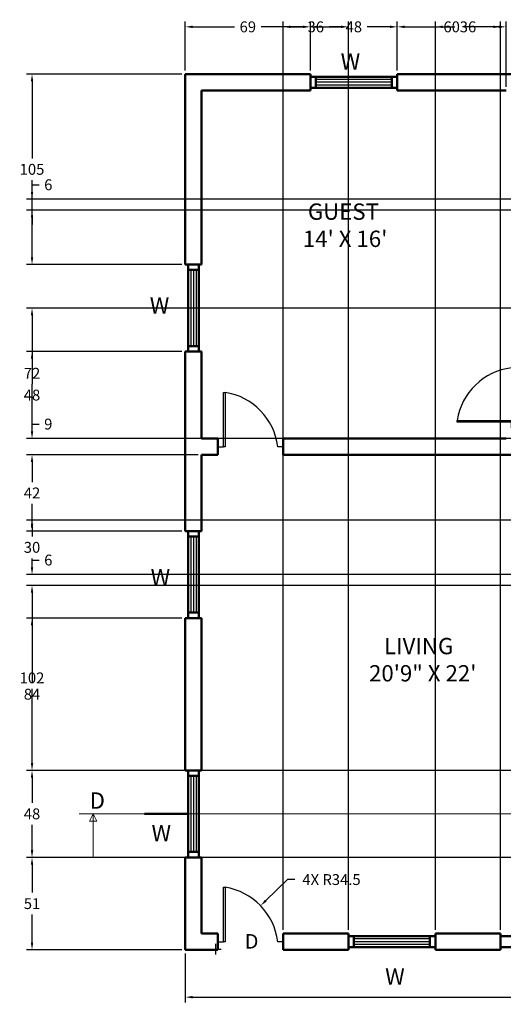
# Model space of a CAD drawing. Units: inches. Extents: x 853 to 2068, y 1026 to 2097.
# Tile 4 of 6: x 1489 to 1756, y 1026 to 1569. Entities that reach past the tile are written whole.
import ezdxf

# ---------------------------------------------------------------- set-up
doc = ezdxf.new("R2010")
doc.units = ezdxf.units.IN
doc.header["$MEASUREMENT"] = 0
for name, color, linetype, lineweight in [('A-ANNO-DIMS', 2, 'Continuous', 18), ('A-ANNO-SYMB', 2, 'Continuous', 18), ('A-ANNO-TEXT', 3, 'Continuous', 18), ('A-AREA-IDEN', 7, 'Continuous', 18), ('A-DOOR', 3, 'Continuous', 25), ('A-GLAZ', 4, 'Continuous', 25), ('A-WALL', 7, 'Continuous', 50)]:
    doc.layers.add(name, color=color, linetype=linetype, lineweight=lineweight)
doc.styles.get("Standard").update_dxf_attribs({"font": 'arial.ttf'})
doc.dimstyles.get("Standard").update_dxf_attribs({"dimtxt": 6, "dimasz": 4, "dimexe": 3, "dimexo": 2, "dimgap": 3, "dimtad": 0, "dimtih": 1, "dimtoh": 1, "dimdec": 0, "dimzin": 0, "dimdsep": 46, "dimlunit": 3, "dimtxsty": 'Standard', "dimcen": 3, "dimadec": 0, "dimazin": 0, "dimtfac": 1, "dimtdec": 0, "dimtofl": 0, "dimtmove": 0, "dimatfit": 3, "dimfxl": 1, "dimtolj": 1, "dimtzin": 0, "dimarcsym": 0})

# ---------------------------------------------------------------- blocks, each defined once
blk = doc.blocks.new('DOOR-D')
for p, q in [((0, 36), (0, 33)), ((0, 33), (30, 33)), ((0, 32), (0, 33)), ((30, 33), (30, 32)), ((30, 32), (0, 32)), ((0, 0), (0, 3))]:
    blk.add_line(p, q)
blk.add_arc((-4.1, 37.26), 34.5, 276.8214, 351.2366)
blk = doc.blocks.new('*D45')
at = {"layer": 'A-ANNO-DIMS', "color": 0, "lineweight": -2, "transparency": 16777216}
for p, q in [((1580.64, 1054.25), (1580.64, 1027.15)), ((1976.64, 1054.25), (1976.64, 1027.15)), ((1584.64, 1030.15), (1769.02, 1030.15)), ((1972.64, 1030.15), (1788.27, 1030.15))]:
    blk.add_line(p, q, dxfattribs=at)
at = {"layer": 'A-ANNO-DIMS', "color": 0, "transparency": 16777216}
for points in [[(1584.64, 1030.82), (1584.64, 1029.48), (1580.64, 1030.15)], [(1972.64, 1030.82), (1972.64, 1029.48), (1976.64, 1030.15)]]:
    blk.add_solid(points, dxfattribs=at)
at = {"layer": 'Defpoints', "color": 0, "transparency": 16777216}
for p in [(1580.64, 1056.25), (1976.64, 1056.25), (1976.64, 1030.15)]:
    blk.add_point(p, dxfattribs=at)
at = {"layer": 'A-ANNO-DIMS', "color": 0, "transparency": 16777216, "insert": (1778.64, 1030.15), "char_height": 6, "attachment_point": 5}
blk.add_mtext('\\A1;396', dxfattribs=at)
blk = doc.blocks.new('*D46')
at = {"layer": 'A-ANNO-DIMS', "color": 0, "lineweight": -2, "transparency": 16777216}
for p, q in [((1634.64, 1067.25), (1634.64, 1568.35)), ((1638.64, 1565.35), (1645.35, 1565.35)), ((1666.64, 1565.35), (1659.94, 1565.35)), ((1670.64, 1067.25), (1670.64, 1568.35))]:
    blk.add_line(p, q, dxfattribs=at)
at = {"layer": 'A-ANNO-DIMS', "color": 0, "transparency": 16777216}
for points in [[(1638.64, 1566.02), (1638.64, 1564.68), (1634.64, 1565.35)], [(1666.64, 1566.02), (1666.64, 1564.68), (1670.64, 1565.35)]]:
    blk.add_solid(points, dxfattribs=at)
at = {"layer": 'Defpoints', "color": 0, "transparency": 16777216}
for p in [(1670.64, 1565.35), (1634.64, 1065.25), (1670.64, 1065.25)]:
    blk.add_point(p, dxfattribs=at)
at = {"layer": 'A-ANNO-DIMS', "color": 0, "transparency": 16777216, "insert": (1652.64, 1565.35), "char_height": 6, "attachment_point": 5}
blk.add_mtext('\\A1;36', dxfattribs=at)
blk = doc.blocks.new('*D47')
at = {"layer": 'A-ANNO-DIMS', "color": 0, "lineweight": -2, "transparency": 16777216}
for p, q in [((1718.64, 1067.25), (1718.64, 1568.35)), ((1722.64, 1565.35), (1729.35, 1565.35)), ((1750.64, 1565.35), (1743.94, 1565.35)), ((1754.64, 1067.25), (1754.64, 1568.35))]:
    blk.add_line(p, q, dxfattribs=at)
at = {"layer": 'A-ANNO-DIMS', "color": 0, "transparency": 16777216}
for points in [[(1722.64, 1566.02), (1722.64, 1564.68), (1718.64, 1565.35)], [(1750.64, 1566.02), (1750.64, 1564.68), (1754.64, 1565.35)]]:
    blk.add_solid(points, dxfattribs=at)
at = {"layer": 'Defpoints', "color": 0, "transparency": 16777216}
for p in [(1754.64, 1565.35), (1718.64, 1065.25), (1754.64, 1065.25)]:
    blk.add_point(p, dxfattribs=at)
at = {"layer": 'A-ANNO-DIMS', "color": 0, "transparency": 16777216, "insert": (1736.64, 1565.35), "char_height": 6, "attachment_point": 5}
blk.add_mtext('\\A1;36', dxfattribs=at)
blk = doc.blocks.new('*D51')
at = {"layer": 'A-ANNO-DIMS', "color": 0, "lineweight": -2, "transparency": 16777216}
for p, q in [((1580.64, 1541.25), (1580.64, 1568.35)), ((1584.64, 1565.35), (1607.82, 1565.35)), ((1645.64, 1565.35), (1622.46, 1565.35)), ((1649.64, 1541.25), (1649.64, 1568.35))]:
    blk.add_line(p, q, dxfattribs=at)
at = {"layer": 'A-ANNO-DIMS', "color": 0, "transparency": 16777216}
for points in [[(1584.64, 1566.02), (1584.64, 1564.68), (1580.64, 1565.35)], [(1645.64, 1566.02), (1645.64, 1564.68), (1649.64, 1565.35)]]:
    blk.add_solid(points, dxfattribs=at)
at = {"layer": 'Defpoints', "color": 0, "transparency": 16777216}
for p in [(1649.64, 1565.35), (1580.64, 1539.25), (1649.64, 1539.25)]:
    blk.add_point(p, dxfattribs=at)
at = {"layer": 'A-ANNO-DIMS', "color": 0, "transparency": 16777216, "insert": (1615.14, 1565.35), "char_height": 6, "attachment_point": 5}
blk.add_mtext('\\A1;69', dxfattribs=at)
blk = doc.blocks.new('*D52')
at = {"layer": 'A-ANNO-DIMS', "color": 0, "lineweight": -2, "transparency": 16777216}
for p, q in [((1649.64, 1541.25), (1649.64, 1568.35)), ((1653.64, 1565.35), (1666.22, 1565.35)), ((1693.64, 1565.35), (1681.07, 1565.35)), ((1697.64, 1541.25), (1697.64, 1568.35))]:
    blk.add_line(p, q, dxfattribs=at)
at = {"layer": 'A-ANNO-DIMS', "color": 0, "transparency": 16777216}
for points in [[(1653.64, 1566.02), (1653.64, 1564.68), (1649.64, 1565.35)], [(1693.64, 1566.02), (1693.64, 1564.68), (1697.64, 1565.35)]]:
    blk.add_solid(points, dxfattribs=at)
at = {"layer": 'Defpoints', "color": 0, "transparency": 16777216}
for p in [(1697.64, 1565.35), (1649.64, 1539.25), (1697.64, 1539.25)]:
    blk.add_point(p, dxfattribs=at)
at = {"layer": 'A-ANNO-DIMS', "color": 0, "transparency": 16777216, "insert": (1673.64, 1565.35), "char_height": 6, "attachment_point": 5}
blk.add_mtext('\\A1;48', dxfattribs=at)
blk = doc.blocks.new('*D53')
at = {"layer": 'A-ANNO-DIMS', "color": 0, "lineweight": -2, "transparency": 16777216}
for p, q in [((1697.64, 1541.25), (1697.64, 1568.35)), ((1701.64, 1565.35), (1720.34, 1565.35)), ((1753.64, 1565.35), (1734.95, 1565.35)), ((1757.64, 1532.25), (1757.64, 1568.35))]:
    blk.add_line(p, q, dxfattribs=at)
at = {"layer": 'A-ANNO-DIMS', "color": 0, "transparency": 16777216}
for points in [[(1701.64, 1566.02), (1701.64, 1564.68), (1697.64, 1565.35)], [(1753.64, 1566.02), (1753.64, 1564.68), (1757.64, 1565.35)]]:
    blk.add_solid(points, dxfattribs=at)
at = {"layer": 'Defpoints', "color": 0, "transparency": 16777216}
for p in [(1757.64, 1565.35), (1697.64, 1539.25), (1757.64, 1530.25)]:
    blk.add_point(p, dxfattribs=at)
at = {"layer": 'A-ANNO-DIMS', "color": 0, "transparency": 16777216, "insert": (1727.64, 1565.35), "char_height": 6, "attachment_point": 5}
blk.add_mtext('\\A1;60', dxfattribs=at)
blk = doc.blocks.new('*D60')
at = {"layer": 'A-ANNO-DIMS', "color": 0, "lineweight": -2, "transparency": 16777216}
for p, q in [((1578.64, 1107.25), (1493.04, 1107.25)), ((1496.04, 1103.25), (1496.04, 1087.81)), ((1496.04, 1060.25), (1496.04, 1075.69)), ((1578.64, 1056.25), (1493.04, 1056.25))]:
    blk.add_line(p, q, dxfattribs=at)
at = {"layer": 'A-ANNO-DIMS', "color": 0, "transparency": 16777216}
for points in [[(1495.38, 1103.25), (1496.71, 1103.25), (1496.04, 1107.25)], [(1495.38, 1060.25), (1496.71, 1060.25), (1496.04, 1056.25)]]:
    blk.add_solid(points, dxfattribs=at)
at = {"layer": 'Defpoints', "color": 0, "transparency": 16777216}
for p in [(1496.04, 1107.25), (1580.64, 1107.25), (1580.64, 1056.25)]:
    blk.add_point(p, dxfattribs=at)
at = {"layer": 'A-ANNO-DIMS', "color": 0, "transparency": 16777216, "insert": (1496.04, 1081.75), "char_height": 6, "attachment_point": 5}
blk.add_mtext('\\A1;51', dxfattribs=at)
blk = doc.blocks.new('*D61')
at = {"layer": 'A-ANNO-DIMS', "color": 0, "lineweight": -2, "transparency": 16777216}
for p, q in [((1578.64, 1239.25), (1493.04, 1239.25)), ((1496.04, 1235.25), (1496.04, 1203.31)), ((1496.04, 1159.25), (1496.04, 1191.19)), ((1578.64, 1155.25), (1493.04, 1155.25))]:
    blk.add_line(p, q, dxfattribs=at)
at = {"layer": 'A-ANNO-DIMS', "color": 0, "transparency": 16777216}
for points in [[(1495.38, 1235.25), (1496.71, 1235.25), (1496.04, 1239.25)], [(1495.38, 1159.25), (1496.71, 1159.25), (1496.04, 1155.25)]]:
    blk.add_solid(points, dxfattribs=at)
at = {"layer": 'Defpoints', "color": 0, "transparency": 16777216}
for p in [(1496.04, 1239.25), (1580.64, 1239.25), (1580.64, 1155.25)]:
    blk.add_point(p, dxfattribs=at)
at = {"layer": 'A-ANNO-DIMS', "color": 0, "transparency": 16777216, "insert": (1496.04, 1197.25), "char_height": 6, "attachment_point": 5}
blk.add_mtext('\\A1;84', dxfattribs=at)
blk = doc.blocks.new('*D62')
at = {"layer": 'A-ANNO-DIMS', "color": 0, "lineweight": -2, "transparency": 16777216}
for p, q in [((1587.64, 1329.25), (1493.04, 1329.25)), ((1496.04, 1325.25), (1496.04, 1314.26)), ((1496.04, 1291.25), (1496.04, 1302.24)), ((1578.64, 1287.25), (1493.04, 1287.25))]:
    blk.add_line(p, q, dxfattribs=at)
at = {"layer": 'A-ANNO-DIMS', "color": 0, "transparency": 16777216}
for points in [[(1495.38, 1325.25), (1496.71, 1325.25), (1496.04, 1329.25)], [(1495.38, 1291.25), (1496.71, 1291.25), (1496.04, 1287.25)]]:
    blk.add_solid(points, dxfattribs=at)
at = {"layer": 'Defpoints', "color": 0, "transparency": 16777216}
for p in [(1496.04, 1329.25), (1589.64, 1329.25), (1580.64, 1287.25)]:
    blk.add_point(p, dxfattribs=at)
at = {"layer": 'A-ANNO-DIMS', "color": 0, "transparency": 16777216, "insert": (1496.04, 1308.25), "char_height": 6, "attachment_point": 5}
blk.add_mtext('\\A1;42', dxfattribs=at)
blk = doc.blocks.new('*D63')
at = {"layer": 'A-ANNO-DIMS', "color": 0, "lineweight": -2, "transparency": 16777216}
for p, q in [((1496.04, 1342.25), (1496.04, 1346.25)), ((1496.04, 1346.25), (1500.04, 1346.25)), ((1587.64, 1338.25), (1493.04, 1338.25)), ((1587.64, 1329.25), (1493.04, 1329.25)), ((1496.04, 1325.25), (1496.04, 1321.25))]:
    blk.add_line(p, q, dxfattribs=at)
at = {"layer": 'A-ANNO-DIMS', "color": 0, "transparency": 16777216}
for points in [[(1495.38, 1342.25), (1496.71, 1342.25), (1496.04, 1338.25)], [(1495.38, 1325.25), (1496.71, 1325.25), (1496.04, 1329.25)]]:
    blk.add_solid(points, dxfattribs=at)
at = {"layer": 'Defpoints', "color": 0, "transparency": 16777216}
for p in [(1496.04, 1338.25), (1589.64, 1338.25), (1589.64, 1329.25)]:
    blk.add_point(p, dxfattribs=at)
at = {"layer": 'A-ANNO-DIMS', "color": 0, "transparency": 16777216, "insert": (1505.01, 1346.25), "char_height": 6, "attachment_point": 5}
blk.add_mtext('\\A1;9', dxfattribs=at)
blk = doc.blocks.new('*D64')
at = {"layer": 'A-ANNO-DIMS', "color": 0, "lineweight": -2, "transparency": 16777216}
for p, q in [((1578.64, 1386.25), (1493.04, 1386.25)), ((1496.04, 1382.25), (1496.04, 1368.31)), ((1496.04, 1342.25), (1496.04, 1356.19)), ((1587.64, 1338.25), (1493.04, 1338.25))]:
    blk.add_line(p, q, dxfattribs=at)
at = {"layer": 'A-ANNO-DIMS', "color": 0, "transparency": 16777216}
for points in [[(1495.38, 1382.25), (1496.71, 1382.25), (1496.04, 1386.25)], [(1495.38, 1342.25), (1496.71, 1342.25), (1496.04, 1338.25)]]:
    blk.add_solid(points, dxfattribs=at)
at = {"layer": 'Defpoints', "color": 0, "transparency": 16777216}
for p in [(1496.04, 1386.25), (1580.64, 1386.25), (1589.64, 1338.25)]:
    blk.add_point(p, dxfattribs=at)
at = {"layer": 'A-ANNO-DIMS', "color": 0, "transparency": 16777216, "insert": (1496.04, 1362.25), "char_height": 6, "attachment_point": 5}
blk.add_mtext('\\A1;48', dxfattribs=at)
blk = doc.blocks.new('*D65')
at = {"layer": 'A-ANNO-DIMS', "color": 0, "lineweight": -2, "transparency": 16777216}
for p, q in [((1578.64, 1539.25), (1493.04, 1539.25)), ((1496.04, 1535.25), (1496.04, 1492.81)), ((1496.04, 1438.25), (1496.04, 1480.69)), ((1578.64, 1434.25), (1493.04, 1434.25))]:
    blk.add_line(p, q, dxfattribs=at)
at = {"layer": 'A-ANNO-DIMS', "color": 0, "transparency": 16777216}
for points in [[(1495.38, 1535.25), (1496.71, 1535.25), (1496.04, 1539.25)], [(1495.38, 1438.25), (1496.71, 1438.25), (1496.04, 1434.25)]]:
    blk.add_solid(points, dxfattribs=at)
at = {"layer": 'Defpoints', "color": 0, "transparency": 16777216}
for p in [(1496.04, 1539.25), (1580.64, 1539.25), (1580.64, 1434.25)]:
    blk.add_point(p, dxfattribs=at)
at = {"layer": 'A-ANNO-DIMS', "color": 0, "transparency": 16777216, "insert": (1496.04, 1486.75), "char_height": 6, "attachment_point": 5}
blk.add_mtext('\\A1;105', dxfattribs=at)
blk = doc.blocks.new('*D67')
at = {"layer": 'A-ANNO-DIMS', "color": 0, "lineweight": -2, "transparency": 16777216}
for p, q in [((1965.64, 1155.25), (1493.04, 1155.25)), ((1496.04, 1151.25), (1496.04, 1137.31)), ((1496.04, 1111.25), (1496.04, 1125.19)), ((1965.64, 1107.25), (1493.04, 1107.25))]:
    blk.add_line(p, q, dxfattribs=at)
at = {"layer": 'A-ANNO-DIMS', "color": 0, "transparency": 16777216}
for points in [[(1495.38, 1151.25), (1496.71, 1151.25), (1496.04, 1155.25)], [(1495.38, 1111.25), (1496.71, 1111.25), (1496.04, 1107.25)]]:
    blk.add_solid(points, dxfattribs=at)
at = {"layer": 'Defpoints', "color": 0, "transparency": 16777216}
for p in [(1496.04, 1155.25), (1967.64, 1155.25), (1967.64, 1107.25)]:
    blk.add_point(p, dxfattribs=at)
at = {"layer": 'A-ANNO-DIMS', "color": 0, "transparency": 16777216, "insert": (1496.04, 1131.25), "char_height": 6, "attachment_point": 5}
blk.add_mtext('\\A1;48', dxfattribs=at)
blk = doc.blocks.new('*D68')
at = {"layer": 'A-ANNO-DIMS', "color": 0, "lineweight": -2, "transparency": 16777216}
for p, q in [((1965.64, 1257.25), (1493.04, 1257.25)), ((1496.04, 1253.25), (1496.04, 1212.31)), ((1496.04, 1159.25), (1496.04, 1200.19)), ((1965.64, 1155.25), (1493.04, 1155.25))]:
    blk.add_line(p, q, dxfattribs=at)
at = {"layer": 'A-ANNO-DIMS', "color": 0, "transparency": 16777216}
for points in [[(1495.38, 1253.25), (1496.71, 1253.25), (1496.04, 1257.25)], [(1495.38, 1159.25), (1496.71, 1159.25), (1496.04, 1155.25)]]:
    blk.add_solid(points, dxfattribs=at)
at = {"layer": 'Defpoints', "color": 0, "transparency": 16777216}
for p in [(1496.04, 1257.25), (1967.64, 1257.25), (1967.64, 1155.25)]:
    blk.add_point(p, dxfattribs=at)
at = {"layer": 'A-ANNO-DIMS', "color": 0, "transparency": 16777216, "insert": (1496.04, 1206.25), "char_height": 6, "attachment_point": 5}
blk.add_mtext('\\A1;102', dxfattribs=at)
blk = doc.blocks.new('*D69')
at = {"layer": 'A-ANNO-DIMS', "color": 0, "lineweight": -2, "transparency": 16777216}
for p, q in [((1496.04, 1267.25), (1496.04, 1271.25)), ((1496.04, 1271.25), (1500.04, 1271.25)), ((1965.64, 1263.25), (1493.04, 1263.25)), ((1965.64, 1257.25), (1493.04, 1257.25)), ((1496.04, 1253.25), (1496.04, 1249.25))]:
    blk.add_line(p, q, dxfattribs=at)
at = {"layer": 'A-ANNO-DIMS', "color": 0, "transparency": 16777216}
for points in [[(1495.38, 1267.25), (1496.71, 1267.25), (1496.04, 1263.25)], [(1495.38, 1253.25), (1496.71, 1253.25), (1496.04, 1257.25)]]:
    blk.add_solid(points, dxfattribs=at)
at = {"layer": 'Defpoints', "color": 0, "transparency": 16777216}
for p in [(1496.04, 1263.25), (1967.64, 1263.25), (1967.64, 1257.25)]:
    blk.add_point(p, dxfattribs=at)
at = {"layer": 'A-ANNO-DIMS', "color": 0, "transparency": 16777216, "insert": (1505.02, 1271.25), "char_height": 6, "attachment_point": 5}
blk.add_mtext('\\A1;6', dxfattribs=at)
blk = doc.blocks.new('*D70')
at = {"layer": 'A-ANNO-DIMS', "color": 0, "lineweight": -2, "transparency": 16777216}
for p, q in [((1965.64, 1410.25), (1493.04, 1410.25)), ((1496.04, 1406.25), (1496.04, 1380.26)), ((1496.04, 1342.25), (1496.04, 1368.24)), ((1965.64, 1338.25), (1493.04, 1338.25))]:
    blk.add_line(p, q, dxfattribs=at)
at = {"layer": 'A-ANNO-DIMS', "color": 0, "transparency": 16777216}
for points in [[(1495.38, 1406.25), (1496.71, 1406.25), (1496.04, 1410.25)], [(1495.38, 1342.25), (1496.71, 1342.25), (1496.04, 1338.25)]]:
    blk.add_solid(points, dxfattribs=at)
at = {"layer": 'Defpoints', "color": 0, "transparency": 16777216}
for p in [(1496.04, 1410.25), (1967.64, 1410.25), (1967.64, 1338.25)]:
    blk.add_point(p, dxfattribs=at)
at = {"layer": 'A-ANNO-DIMS', "color": 0, "transparency": 16777216, "insert": (1496.04, 1374.25), "char_height": 6, "attachment_point": 5}
blk.add_mtext('\\A1;72', dxfattribs=at)
blk = doc.blocks.new('*D71')
at = {"layer": 'A-ANNO-DIMS', "color": 0, "lineweight": -2, "transparency": 16777216}
for p, q in [((1496.04, 1474.25), (1496.04, 1478.25)), ((1496.04, 1478.25), (1500.04, 1478.25)), ((1836.64, 1470.25), (1493.04, 1470.25)), ((1836.64, 1464.25), (1493.04, 1464.25)), ((1496.04, 1460.25), (1496.04, 1456.25))]:
    blk.add_line(p, q, dxfattribs=at)
at = {"layer": 'A-ANNO-DIMS', "color": 0, "transparency": 16777216}
for points in [[(1495.38, 1474.25), (1496.71, 1474.25), (1496.04, 1470.25)], [(1495.38, 1460.25), (1496.71, 1460.25), (1496.04, 1464.25)]]:
    blk.add_solid(points, dxfattribs=at)
at = {"layer": 'Defpoints', "color": 0, "transparency": 16777216}
for p in [(1496.04, 1470.25), (1838.64, 1470.25), (1838.64, 1464.25)]:
    blk.add_point(p, dxfattribs=at)
at = {"layer": 'A-ANNO-DIMS', "color": 0, "transparency": 16777216, "insert": (1505.02, 1478.25), "char_height": 6, "attachment_point": 5}
blk.add_mtext('\\A1;6', dxfattribs=at)
blk = doc.blocks.new('*D75')
at = {"layer": 'A-ANNO-DIMS', "color": 0, "lineweight": -2, "transparency": 16777216}
for p, q in [((1866.64, 1293.25), (1493.04, 1293.25)), ((1496.04, 1289.25), (1496.04, 1284.32)), ((1496.04, 1267.25), (1496.04, 1272.19)), ((1866.64, 1263.25), (1493.04, 1263.25))]:
    blk.add_line(p, q, dxfattribs=at)
at = {"layer": 'A-ANNO-DIMS', "color": 0, "transparency": 16777216}
for points in [[(1495.38, 1289.25), (1496.71, 1289.25), (1496.04, 1293.25)], [(1495.38, 1267.25), (1496.71, 1267.25), (1496.04, 1263.25)]]:
    blk.add_solid(points, dxfattribs=at)
at = {"layer": 'Defpoints', "color": 0, "transparency": 16777216}
for p in [(1496.04, 1293.25), (1868.64, 1293.25), (1868.64, 1263.25)]:
    blk.add_point(p, dxfattribs=at)
at = {"layer": 'A-ANNO-DIMS', "color": 0, "transparency": 16777216, "insert": (1496.04, 1278.25), "char_height": 6, "attachment_point": 5}
blk.add_mtext('\\A1;30', dxfattribs=at)
blk = doc.blocks.new('*D118')
at = {"layer": 'A-ANNO-DIMS', "color": 0, "lineweight": -2, "transparency": 16777216}
for p, q in [((1637.07, 1095.02), (1625.07, 1083.41)), ((1641.07, 1095.02), (1637.07, 1095.02)), ((1597.39, 1053.65), (1597.39, 1059.65)), ((1594.39, 1056.65), (1600.39, 1056.65))]:
    blk.add_line(p, q, dxfattribs=at)
at = {"layer": 'A-ANNO-DIMS', "color": 0, "transparency": 16777216}
blk.add_solid([(1624.6, 1083.89), (1625.53, 1082.93), (1622.19, 1080.63)], dxfattribs=at)
at = {"layer": 'Defpoints', "color": 0, "transparency": 16777216}
for p in [(1622.19, 1080.63), (1597.39, 1056.65)]:
    blk.add_point(p, dxfattribs=at)
at = {"layer": 'A-ANNO-DIMS', "color": 0, "transparency": 16777216, "insert": (1661.33, 1095.02), "char_height": 6, "attachment_point": 5}
blk.add_mtext('\\A1;4X R34.5', dxfattribs=at)

msp = doc.modelspace()

# ---------------------------------------------------------------- linework, layer by layer
at = {"layer": 'A-ANNO-SYMB'}
for p, q in [((1522.142, 1131.2513), (2035.142, 1131.2513)), ((1527.7311, 1127.2513), (1529.7311, 1131.2513)), ((1529.7311, 1131.2513), (1529.7311, 1107.2513)), ((1529.7311, 1131.2513), (1529.7311, 1127.2513)), ((1531.7311, 1127.2513), (1529.7311, 1131.2513)), ((1529.7311, 1131.2513), (1529.7311, 1127.2513)), ((1529.7311, 1127.2513), (1527.7311, 1127.2513)), ((1529.7311, 1127.2513), (1531.7311, 1127.2513))]:
    msp.add_line(p, q, dxfattribs=at)
at = {"layer": 'A-GLAZ'}
for p, q in [((1694.642, 1536.2513), (1652.642, 1536.2513)), ((1694.642, 1534.7513), (1652.642, 1534.7513)), ((1694.642, 1533.2513), (1652.642, 1533.2513)), ((1583.642, 1431.2513), (1583.642, 1389.2513)), ((1585.142, 1431.2513), (1585.142, 1389.2513)), ((1586.642, 1431.2513), (1586.642, 1389.2513)), ((1583.642, 1284.2513), (1583.642, 1242.2513)), ((1585.142, 1284.2513), (1585.142, 1242.2513)), ((1586.642, 1284.2513), (1586.642, 1242.2513)), ((1583.642, 1152.2513), (1583.642, 1110.2513)), ((1585.142, 1152.2513), (1585.142, 1110.2513)), ((1586.642, 1152.2513), (1586.642, 1110.2513)), ((1715.642, 1062.2513), (1673.642, 1062.2513)), ((1715.642, 1060.7513), (1673.642, 1060.7513)), ((1715.642, 1059.2513), (1673.642, 1059.2513))]:
    msp.add_line(p, q, dxfattribs=at)
at = {"layer": 'A-WALL'}
for p, q in [((1580.642, 1434.2513), (1580.642, 1539.2513)), ((1580.642, 1539.2513), (1649.642, 1539.2513)), ((1649.642, 1539.2513), (1649.642, 1530.2513)), ((1697.642, 1537.7513), (1649.642, 1537.7513)), ((1652.642, 1537.7513), (1652.642, 1531.7513)), ((1694.642, 1537.7513), (1694.642, 1531.7513)), ((1697.642, 1539.2513), (1790.642, 1539.2513)), ((1697.642, 1539.2513), (1697.642, 1530.2513)), ((1697.642, 1531.7513), (1649.642, 1531.7513)), ((1589.642, 1434.2513), (1589.642, 1530.2513)), ((1589.642, 1530.2513), (1649.642, 1530.2513)), ((1589.642, 1530.2513), (1649.642, 1530.2513)), ((1589.642, 1434.2513), (1589.642, 1530.2513)), ((1697.642, 1530.2513), (1757.642, 1530.2513)), ((1697.642, 1530.2513), (1757.642, 1530.2513)), ((1580.642, 1434.2513), (1589.642, 1434.2513)), ((1582.142, 1434.2513), (1582.142, 1386.2513)), ((1588.142, 1434.2513), (1588.142, 1386.2513)), ((1582.142, 1431.2513), (1588.142, 1431.2513)), ((1580.642, 1287.2513), (1580.642, 1386.2513)), ((1580.642, 1386.2513), (1589.642, 1386.2513)), ((1582.142, 1389.2513), (1588.142, 1389.2513)), ((1589.642, 1338.2513), (1589.642, 1386.2513)), ((1598.642, 1338.2513), (1589.642, 1338.2513)), ((1598.642, 1338.2513), (1598.642, 1329.2513)), ((1757.642, 1338.2513), (1634.642, 1338.2513)), ((1634.642, 1338.2513), (1634.642, 1329.2513)), ((1589.642, 1287.2513), (1589.642, 1329.2513)), ((1598.642, 1329.2513), (1589.642, 1329.2513)), ((1589.642, 1329.2513), (1589.642, 1287.2513)), ((1769.642, 1329.2513), (1634.642, 1329.2513)), ((1580.642, 1287.2513), (1589.642, 1287.2513)), ((1582.142, 1287.2513), (1582.142, 1239.2513)), ((1588.142, 1287.2513), (1588.142, 1239.2513)), ((1582.142, 1284.2513), (1588.142, 1284.2513)), ((1580.642, 1155.2513), (1580.642, 1239.2513)), ((1580.642, 1239.2513), (1589.642, 1239.2513)), ((1582.142, 1242.2513), (1588.142, 1242.2513)), ((1589.642, 1155.2513), (1589.642, 1239.2513)), ((1589.642, 1239.2513), (1589.642, 1155.2513)), ((1580.642, 1155.2513), (1589.642, 1155.2513)), ((1582.142, 1155.2513), (1582.142, 1107.2513)), ((1582.142, 1152.2513), (1588.142, 1152.2513)), ((1588.142, 1155.2513), (1588.142, 1107.2513)), ((1582.142, 1131.2513), (1558.142, 1131.2513)), ((1582.142, 1110.2513), (1588.142, 1110.2513)), ((1580.642, 1056.2513), (1580.642, 1107.2513)), ((1580.642, 1107.2513), (1589.642, 1107.2513)), ((1589.642, 1065.2513), (1589.642, 1107.2513)), ((1589.642, 1107.2513), (1589.642, 1065.2513)), ((1589.642, 1065.2513), (1598.642, 1065.2513)), ((1598.642, 1065.2513), (1598.642, 1056.2513)), ((1634.642, 1065.2513), (1670.642, 1065.2513)), ((1634.642, 1065.2513), (1634.642, 1056.2513)), ((1670.642, 1065.2513), (1670.642, 1056.2513)), ((1718.642, 1065.2513), (1754.642, 1065.2513)), ((1718.642, 1065.2513), (1718.642, 1056.2513)), ((1718.642, 1065.2513), (1718.642, 1056.2513)), ((1754.642, 1065.2513), (1754.642, 1056.2513)), ((1754.642, 1065.2513), (1754.642, 1056.2513)), ((1718.642, 1063.7513), (1670.642, 1063.7513)), ((1673.642, 1063.7513), (1673.642, 1057.7513)), ((1715.642, 1063.7513), (1715.642, 1057.7513)), ((1802.642, 1063.7513), (1754.642, 1063.7513)), ((1580.642, 1056.2513), (1598.642, 1056.2513)), ((1634.642, 1056.2513), (1670.642, 1056.2513)), ((1718.642, 1057.7513), (1670.642, 1057.7513)), ((1718.642, 1056.2513), (1754.642, 1056.2513)), ((1802.642, 1057.7513), (1754.642, 1057.7513))]:
    msp.add_line(p, q, dxfattribs=at)

# ---------------------------------------------------------------- block references
at = {"layer": 'A-DOOR'}
for p, rotation in [((1760.642, 1380.2515), 180), ((1634.6423, 1333.7513), 89.9999999999993), ((1634.6423, 1060.7513), 89.99999999999972)]:
    msp.add_blockref('DOOR-D', p, dxfattribs=dict(at, rotation=rotation))

# ---------------------------------------------------------------- texts
at = {"layer": 'A-ANNO-TEXT', "attachment_point": 1}
for s, insert, char_height in [('W', (1666.3723, 1550.7548), 9), ('W', (1561.0183, 1416.2013), 9), ('W', (1561.5021, 1266.2835), 9), ('{\\fArial|b1|i0|c0|p34;D}', (1527.8294, 1143.0903), 9), ('W', (1561.9855, 1125.1936), 9), ('D', (1613.4807, 1064.9345), 8), ('W', (1690.9263, 1046.0098), 9)]:
    msp.add_mtext_dynamic_manual_height_columns(s, width=85.037544, gutter_width=1, heights=[0], dxfattribs=dict(at, insert=insert, char_height=char_height))
at = {"layer": 'A-AREA-IDEN', "char_height": 9, "attachment_point": 1}
for s, insert in [("      GUEST\\P     14' X 16'", (1631.7658, 1467.9284)), ('   LIVING\\P20\'9" X 22\'', (1682.0338, 1228.2964))]:
    msp.add_mtext_dynamic_manual_height_columns(s, width=85.037544, gutter_width=1, heights=[0], dxfattribs=dict(at, insert=insert))

# ---------------------------------------------------------------- dimensions: what is measured, and where the dimension line sits
at = {"layer": 'A-ANNO-DIMS'}
for base, p1, p2, picture, middle in [((1649.642, 1565.3513), (1580.642, 1539.2513), (1649.642, 1539.2513), '*D51', (1615.142, 1565.3513)), ((1670.642, 1565.3513), (1634.642, 1065.2513), (1670.642, 1065.2513), '*D46', (1652.642, 1565.3513)), ((1697.642, 1565.3513), (1649.642, 1539.2513), (1697.642, 1539.2513), '*D52', (1673.642, 1565.3513)), ((1757.642, 1565.3513), (1697.642, 1539.2513), (1757.642, 1530.2513), '*D53', (1727.642, 1565.3513)), ((1754.642, 1565.3513), (1718.642, 1065.2513), (1754.642, 1065.2513), '*D47', (1736.642, 1565.3513)), ((1976.642, 1030.1513), (1580.642, 1056.2513), (1976.642, 1056.2513), '*D45', (1778.642, 1030.1513))]:
    dim = msp.add_linear_dim(base=base, p1=p1, p2=p2, dimstyle='Standard', override={"dimdec": 0, "dimlfac": 1, "dimrnd": 0, "dimzin": 0, "dimdsep": 46, "dimlunit": 2}, dxfattribs=at)
    dim.commit()
    dim.dimension.update_dxf_attribs({"geometry": picture, "text_midpoint": middle})
for base, p1, p2, picture, middle in [((1496.042, 1539.2513), (1580.642, 1434.2513), (1580.642, 1539.2513), '*D65', (1496.042, 1486.7513)), ((1496.042, 1470.2513), (1838.642, 1464.2513), (1838.642, 1470.2513), '*D71', (1505.0229, 1478.2513)), ((1496.042, 1410.2513), (1967.642, 1338.2513), (1967.642, 1410.2513), '*D70', (1496.042, 1374.2513)), ((1496.042, 1386.2513), (1589.642, 1338.2513), (1580.642, 1386.2513), '*D64', (1496.042, 1362.2513)), ((1496.042, 1338.2513), (1589.642, 1329.2513), (1589.642, 1338.2513), '*D63', (1505.0148, 1346.2513)), ((1496.042, 1329.2513), (1580.642, 1287.2513), (1589.642, 1329.2513), '*D62', (1496.042, 1308.2513)), ((1496.042, 1293.2513), (1868.642, 1263.2513), (1868.642, 1293.2513), '*D75', (1496.042, 1278.2513)), ((1496.042, 1263.2513), (1967.642, 1257.2513), (1967.642, 1263.2513), '*D69', (1505.0229, 1271.2513)), ((1496.042, 1257.2513), (1967.642, 1155.2513), (1967.642, 1257.2513), '*D68', (1496.042, 1206.2513)), ((1496.042, 1239.2513), (1580.642, 1155.2513), (1580.642, 1239.2513), '*D61', (1496.042, 1197.2513)), ((1496.042, 1155.2513), (1967.642, 1107.2513), (1967.642, 1155.2513), '*D67', (1496.042, 1131.2513)), ((1496.042, 1107.2513), (1580.642, 1056.2513), (1580.642, 1107.2513), '*D60', (1496.042, 1081.7513))]:
    dim = msp.add_linear_dim(base=base, p1=p1, p2=p2, angle=90, dimstyle='Standard', override={"dimdec": 0, "dimlfac": 1, "dimrnd": 0, "dimzin": 0, "dimdsep": 46, "dimlunit": 2}, dxfattribs=at)
    dim.commit()
    dim.dimension.update_dxf_attribs({"geometry": picture, "text_midpoint": middle})
dim = msp.add_radius_dim(center=(1597.3857, 1056.6535), mpoint=(1622.1912, 1080.6322), text='4X <>', dimstyle='Standard', override={"dimdec": 1, "dimlfac": 1, "dimrnd": 0, "dimzin": 0, "dimdsep": 46, "dimlunit": 2}, dxfattribs=at)
dim.commit()
dim.dimension.update_dxf_attribs({"geometry": '*D118', "text_midpoint": (1661.3275, 1095.0194), "dimtype": 164})

doc.saveas('drawing.dxf')
